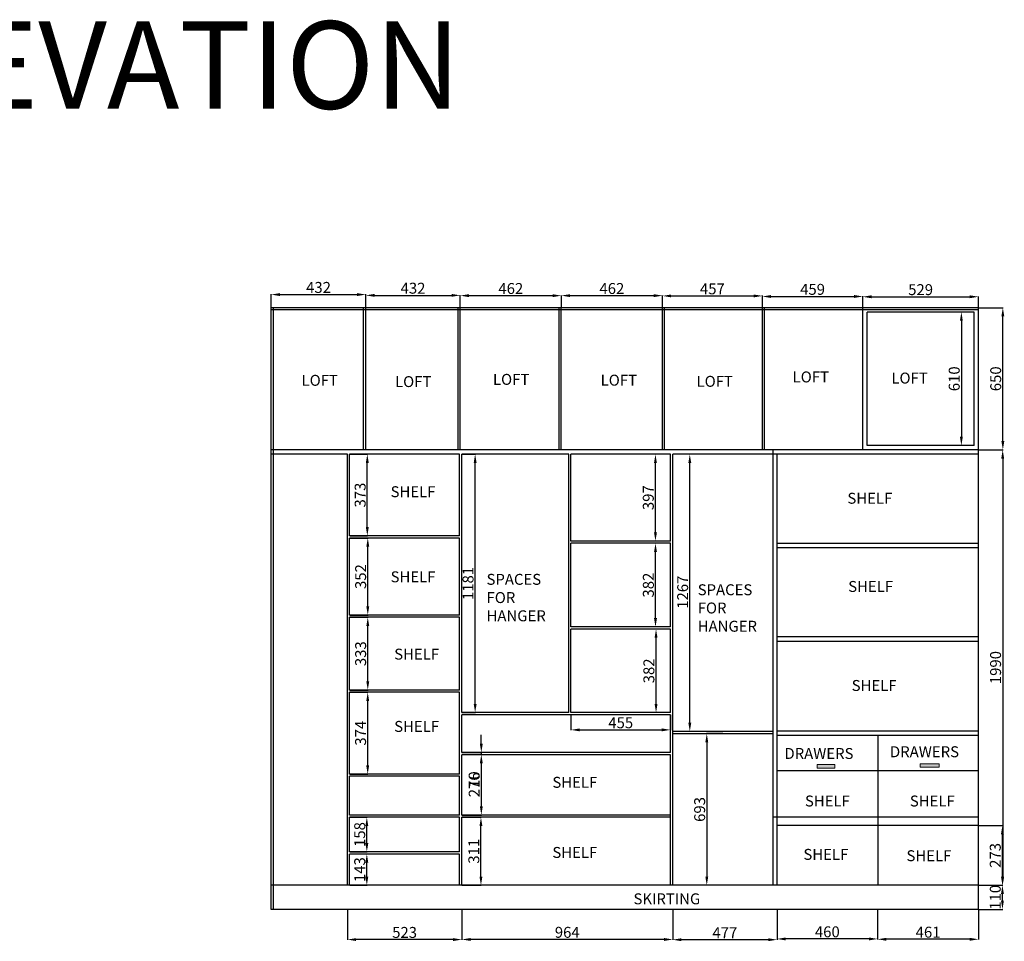
# Model space of a CAD drawing. Units: millimetres. Extents: x 46070 to 59439, y 6883 to 14761.
# Tile 5 of 5: x 54938 to 59439, y 10549 to 14761. Entities that reach past the tile are written whole.
import ezdxf

# ---------------------------------------------------------------- set-up
doc = ezdxf.new("R2010")
doc.units = ezdxf.units.MM
for name, color, linetype, lineweight in [('A-ANNO-DIMS', 2, 'Continuous', 18), ('A-ANNO-TEXT', 7, 'Continuous', 18), ('A-ELEV', 7, 'Continuous', 25), ('A-ELEV-PATT', 8, 'Continuous', 13), ('A-FURN-HDWR', 4, 'Continuous', 18)]:
    doc.layers.add(name, color=color, linetype=linetype, lineweight=lineweight)
doc.styles.get("Standard").update_dxf_attribs({"font": 'arial.ttf'})
doc.dimstyles.new('ISO-25', dxfattribs={"dimtxt": 50, "dimasz": 40, "dimexe": 1.25, "dimexo": 0.625, "dimtad": 1, "dimtxsty": 'Standard', "dimcen": 2.5, "dimadec": 0, "dimazin": 0, "dimtfac": 1, "dimtmove": 0, "dimatfit": 3, "dimfxl": 1, "dimarcsym": 0})

# ---------------------------------------------------------------- blocks, each defined once
blk = doc.blocks.new('*D34')
at = {"layer": 'A-ANNO-DIMS', "color": 0, "lineweight": -2, "transparency": 16777216}
for p, q in [((59321.5, 10805), (59431.6, 10805)), ((59430.3, 10735), (59430.3, 10765)), ((59321.5, 10695), (59431.6, 10695))]:
    blk.add_line(p, q, dxfattribs=at)
at = {"layer": 'A-ANNO-DIMS', "color": 0, "transparency": 16777216}
for points in [[(59423.7, 10765), (59437, 10765), (59430.3, 10805)], [(59423.7, 10735), (59437, 10735), (59430.3, 10695)]]:
    blk.add_solid(points, dxfattribs=at)
at = {"layer": 'Defpoints', "color": 0, "transparency": 16777216}
for p in [(59320.9, 10805), (59430.3, 10805), (59320.9, 10695)]:
    blk.add_point(p, dxfattribs=at)
at = {"layer": 'A-ANNO-DIMS', "color": 0, "transparency": 16777216, "insert": (59404.2, 10750), "char_height": 50, "attachment_point": 5, "rotation": 90}
blk.add_mtext('110', dxfattribs=at)
blk = doc.blocks.new('*D35')
at = {"layer": 'A-ANNO-DIMS', "color": 0, "lineweight": -2, "transparency": 16777216}
for p, q in [((59321.5, 11078), (59431.6, 11078)), ((59430.4, 10845), (59430.4, 11038)), ((59321.5, 10805), (59431.6, 10805))]:
    blk.add_line(p, q, dxfattribs=at)
at = {"layer": 'A-ANNO-DIMS', "color": 0, "transparency": 16777216}
for points in [[(59423.7, 11038), (59437, 11038), (59430.4, 11078)], [(59423.7, 10845), (59437, 10845), (59430.4, 10805)]]:
    blk.add_solid(points, dxfattribs=at)
at = {"layer": 'Defpoints', "color": 0, "transparency": 16777216}
for p in [(59320.9, 11078), (59430.4, 11078), (59320.9, 10805)]:
    blk.add_point(p, dxfattribs=at)
at = {"layer": 'A-ANNO-DIMS', "color": 0, "transparency": 16777216, "insert": (59404.2, 10941.5), "char_height": 50, "attachment_point": 5, "rotation": 90}
blk.add_mtext('273', dxfattribs=at)
blk = doc.blocks.new('*D36')
at = {"layer": 'A-ANNO-DIMS', "color": 0, "lineweight": -2, "transparency": 16777216}
for p, q in [((59321.5, 12795), (59432.9, 12795)), ((59431.6, 12755), (59431.6, 10845)), ((59321.5, 10805), (59432.9, 10805))]:
    blk.add_line(p, q, dxfattribs=at)
at = {"layer": 'A-ANNO-DIMS', "color": 0, "transparency": 16777216}
for points in [[(59424.9, 12755), (59438.3, 12755), (59431.6, 12795)], [(59424.9, 10845), (59438.3, 10845), (59431.6, 10805)]]:
    blk.add_solid(points, dxfattribs=at)
at = {"layer": 'Defpoints', "color": 0, "transparency": 16777216}
for p in [(59320.9, 12795), (59320.9, 10805), (59431.6, 10805)]:
    blk.add_point(p, dxfattribs=at)
at = {"layer": 'A-ANNO-DIMS', "color": 0, "transparency": 16777216, "insert": (59405.5, 11800), "char_height": 50, "attachment_point": 5, "rotation": 90}
blk.add_mtext('1990', dxfattribs=at)
blk = doc.blocks.new('*D37')
at = {"layer": 'A-ANNO-DIMS', "color": 0, "lineweight": -2, "transparency": 16777216}
for p, q in [((58859.9, 10694.3), (58859.9, 10556.8)), ((59320.9, 10694.3), (59320.9, 10556.8)), ((59280.9, 10558.1), (58899.9, 10558.1))]:
    blk.add_line(p, q, dxfattribs=at)
at = {"layer": 'A-ANNO-DIMS', "color": 0, "transparency": 16777216}
for points in [[(58899.9, 10564.8), (58899.9, 10551.4), (58859.9, 10558.1)], [(59280.9, 10564.8), (59280.9, 10551.4), (59320.9, 10558.1)]]:
    blk.add_solid(points, dxfattribs=at)
at = {"layer": 'Defpoints', "color": 0, "transparency": 16777216}
for p in [(58859.9, 10695), (59320.9, 10695), (58859.9, 10558.1)]:
    blk.add_point(p, dxfattribs=at)
at = {"layer": 'A-ANNO-DIMS', "color": 0, "transparency": 16777216, "insert": (59090.4, 10584.2), "char_height": 50, "attachment_point": 5}
blk.add_mtext('461', dxfattribs=at)
blk = doc.blocks.new('*D38')
at = {"layer": 'A-ANNO-DIMS', "color": 0, "lineweight": -2, "transparency": 16777216}
for p, q in [((58399.9, 10694.3), (58399.9, 10558.4)), ((58859.9, 10694.3), (58859.9, 10558.4)), ((58819.9, 10559.6), (58439.9, 10559.6))]:
    blk.add_line(p, q, dxfattribs=at)
at = {"layer": 'A-ANNO-DIMS', "color": 0, "transparency": 16777216}
for points in [[(58439.9, 10566.3), (58439.9, 10553), (58399.9, 10559.6)], [(58819.9, 10566.3), (58819.9, 10553), (58859.9, 10559.6)]]:
    blk.add_solid(points, dxfattribs=at)
at = {"layer": 'Defpoints', "color": 0, "transparency": 16777216}
for p in [(58399.9, 10695), (58859.9, 10695), (58399.9, 10559.6)]:
    blk.add_point(p, dxfattribs=at)
at = {"layer": 'A-ANNO-DIMS', "color": 0, "transparency": 16777216, "insert": (58629.9, 10585.8), "char_height": 50, "attachment_point": 5}
blk.add_mtext('460', dxfattribs=at)
blk = doc.blocks.new('*D39')
at = {"layer": 'A-ANNO-DIMS', "color": 0, "lineweight": -2, "transparency": 16777216}
for p, q in [((57922.9, 10694.3), (57922.9, 10554.9)), ((58399.9, 10694.3), (58399.9, 10554.9)), ((58359.9, 10556.1), (57962.9, 10556.1))]:
    blk.add_line(p, q, dxfattribs=at)
at = {"layer": 'A-ANNO-DIMS', "color": 0, "transparency": 16777216}
for points in [[(57962.9, 10562.8), (57962.9, 10549.4), (57922.9, 10556.1)], [(58359.9, 10562.8), (58359.9, 10549.4), (58399.9, 10556.1)]]:
    blk.add_solid(points, dxfattribs=at)
at = {"layer": 'Defpoints', "color": 0, "transparency": 16777216}
for p in [(57922.9, 10695), (58399.9, 10695), (57922.9, 10556.1)]:
    blk.add_point(p, dxfattribs=at)
at = {"layer": 'A-ANNO-DIMS', "color": 0, "transparency": 16777216, "insert": (58161.4, 10581.7), "char_height": 50, "attachment_point": 5}
blk.add_mtext('477', dxfattribs=at)
blk = doc.blocks.new('*D40')
at = {"layer": 'A-ANNO-DIMS', "color": 0, "lineweight": -2, "transparency": 16777216}
for p, q in [((56958.9, 10694.3), (56958.9, 10556.1)), ((57922.9, 10694.3), (57922.9, 10556.1)), ((57882.9, 10557.3), (56998.9, 10557.3))]:
    blk.add_line(p, q, dxfattribs=at)
at = {"layer": 'A-ANNO-DIMS', "color": 0, "transparency": 16777216}
for points in [[(56998.9, 10564), (56998.9, 10550.6), (56958.9, 10557.3)], [(57882.9, 10564), (57882.9, 10550.6), (57922.9, 10557.3)]]:
    blk.add_solid(points, dxfattribs=at)
at = {"layer": 'Defpoints', "color": 0, "transparency": 16777216}
for p in [(56958.9, 10695), (57922.9, 10695), (56958.9, 10557.3)]:
    blk.add_point(p, dxfattribs=at)
at = {"layer": 'A-ANNO-DIMS', "color": 0, "transparency": 16777216, "insert": (57440.9, 10583.5), "char_height": 50, "attachment_point": 5}
blk.add_mtext('964', dxfattribs=at)
blk = doc.blocks.new('*D41')
at = {"layer": 'A-ANNO-DIMS', "color": 0, "lineweight": -2, "transparency": 16777216}
for p, q in [((56435.9, 10694.3), (56435.9, 10555.5)), ((56958.9, 10694.3), (56958.9, 10555.5)), ((56918.9, 10556.8), (56475.9, 10556.8))]:
    blk.add_line(p, q, dxfattribs=at)
at = {"layer": 'A-ANNO-DIMS', "color": 0, "transparency": 16777216}
for points in [[(56475.9, 10563.4), (56475.9, 10550.1), (56435.9, 10556.8)], [(56918.9, 10563.4), (56918.9, 10550.1), (56958.9, 10556.8)]]:
    blk.add_solid(points, dxfattribs=at)
at = {"layer": 'Defpoints', "color": 0, "transparency": 16777216}
for p in [(56435.9, 10695), (56958.9, 10695), (56435.9, 10556.8)]:
    blk.add_point(p, dxfattribs=at)
at = {"layer": 'A-ANNO-DIMS', "color": 0, "transparency": 16777216, "insert": (56697.4, 10583), "char_height": 50, "attachment_point": 5}
blk.add_mtext('523', dxfattribs=at)
blk = doc.blocks.new('*D43')
at = {"layer": 'A-ANNO-DIMS', "color": 0, "lineweight": -2, "transparency": 16777216}
for p, q in [((59321.5, 13445), (59433.5, 13445)), ((59432.3, 12835), (59432.3, 13405)), ((59321.5, 12795), (59433.5, 12795))]:
    blk.add_line(p, q, dxfattribs=at)
at = {"layer": 'A-ANNO-DIMS', "color": 0, "transparency": 16777216}
for points in [[(59425.6, 13405), (59438.9, 13405), (59432.3, 13445)], [(59425.6, 12835), (59438.9, 12835), (59432.3, 12795)]]:
    blk.add_solid(points, dxfattribs=at)
at = {"layer": 'Defpoints', "color": 0, "transparency": 16777216}
for p in [(59320.9, 13445), (59432.3, 13445), (59320.9, 12795)]:
    blk.add_point(p, dxfattribs=at)
at = {"layer": 'A-ANNO-DIMS', "color": 0, "transparency": 16777216, "insert": (59406.1, 13120), "char_height": 50, "attachment_point": 5, "rotation": 90}
blk.add_mtext('650', dxfattribs=at)
blk = doc.blocks.new('*D44')
at = {"layer": 'A-ANNO-DIMS', "color": 0, "lineweight": -2, "transparency": 16777216}
for p, q in [((59257.7, 13425), (59241.4, 13425)), ((59242.7, 13385), (59242.7, 12855)), ((59257.7, 12815), (59241.4, 12815))]:
    blk.add_line(p, q, dxfattribs=at)
at = {"layer": 'A-ANNO-DIMS', "color": 0, "transparency": 16777216}
for points in [[(59236, 13385), (59249.3, 13385), (59242.7, 13425)], [(59236, 12855), (59249.3, 12855), (59242.7, 12815)]]:
    blk.add_solid(points, dxfattribs=at)
at = {"layer": 'Defpoints', "color": 0, "transparency": 16777216}
for p in [(59258.4, 13425), (59242.7, 12815), (59258.4, 12815)]:
    blk.add_point(p, dxfattribs=at)
at = {"layer": 'A-ANNO-DIMS', "color": 0, "transparency": 16777216, "insert": (59216.5, 13120), "char_height": 50, "attachment_point": 5, "rotation": 90}
blk.add_mtext('610', dxfattribs=at)
blk = doc.blocks.new('*D45')
at = {"layer": 'A-ANNO-DIMS', "color": 0, "lineweight": -2, "transparency": 16777216}
for p, q in [((56087.9, 13445.6), (56087.9, 13506.1)), ((56127.9, 13504.9), (56479.9, 13504.9)), ((56519.9, 13445.6), (56519.9, 13506.1))]:
    blk.add_line(p, q, dxfattribs=at)
at = {"layer": 'A-ANNO-DIMS', "color": 0, "transparency": 16777216}
for points in [[(56127.9, 13511.6), (56127.9, 13498.2), (56087.9, 13504.9)], [(56479.9, 13511.6), (56479.9, 13498.2), (56519.9, 13504.9)]]:
    blk.add_solid(points, dxfattribs=at)
at = {"layer": 'Defpoints', "color": 0, "transparency": 16777216}
for p in [(56519.9, 13504.9), (56087.9, 13445), (56519.9, 13445)]:
    blk.add_point(p, dxfattribs=at)
at = {"layer": 'A-ANNO-DIMS', "color": 0, "transparency": 16777216, "insert": (56303.9, 13531.1), "char_height": 50, "attachment_point": 5}
blk.add_mtext('432', dxfattribs=at)
blk = doc.blocks.new('*D46')
at = {"layer": 'A-ANNO-DIMS', "color": 0, "lineweight": -2, "transparency": 16777216}
for p, q in [((56519.9, 13445.6), (56519.9, 13502.6)), ((56559.9, 13501.3), (56911.9, 13501.3)), ((56951.9, 13445.6), (56951.9, 13502.6))]:
    blk.add_line(p, q, dxfattribs=at)
at = {"layer": 'A-ANNO-DIMS', "color": 0, "transparency": 16777216}
for points in [[(56559.9, 13508), (56559.9, 13494.7), (56519.9, 13501.3)], [(56911.9, 13508), (56911.9, 13494.7), (56951.9, 13501.3)]]:
    blk.add_solid(points, dxfattribs=at)
at = {"layer": 'Defpoints', "color": 0, "transparency": 16777216}
for p in [(56951.9, 13501.3), (56519.9, 13445), (56951.9, 13445)]:
    blk.add_point(p, dxfattribs=at)
at = {"layer": 'A-ANNO-DIMS', "color": 0, "transparency": 16777216, "insert": (56735.9, 13527.5), "char_height": 50, "attachment_point": 5}
blk.add_mtext('432', dxfattribs=at)
blk = doc.blocks.new('*D47')
at = {"layer": 'A-ANNO-DIMS', "color": 0, "lineweight": -2, "transparency": 16777216}
for p, q in [((56951.9, 13445.6), (56951.9, 13501.3)), ((56991.9, 13500), (57373.9, 13500)), ((57413.9, 13445.6), (57413.9, 13501.3))]:
    blk.add_line(p, q, dxfattribs=at)
at = {"layer": 'A-ANNO-DIMS', "color": 0, "transparency": 16777216}
for points in [[(56991.9, 13506.7), (56991.9, 13493.4), (56951.9, 13500)], [(57373.9, 13506.7), (57373.9, 13493.4), (57413.9, 13500)]]:
    blk.add_solid(points, dxfattribs=at)
at = {"layer": 'Defpoints', "color": 0, "transparency": 16777216}
for p in [(57413.9, 13500), (56951.9, 13445), (57413.9, 13445)]:
    blk.add_point(p, dxfattribs=at)
at = {"layer": 'A-ANNO-DIMS', "color": 0, "transparency": 16777216, "insert": (57182.9, 13526.2), "char_height": 50, "attachment_point": 5}
blk.add_mtext('462', dxfattribs=at)
blk = doc.blocks.new('*D48')
at = {"layer": 'A-ANNO-DIMS', "color": 0, "lineweight": -2, "transparency": 16777216}
for p, q in [((57413.9, 13445.6), (57413.9, 13501.3)), ((57453.9, 13500.1), (57835.9, 13500.1)), ((57875.9, 13445.6), (57875.9, 13501.3))]:
    blk.add_line(p, q, dxfattribs=at)
at = {"layer": 'A-ANNO-DIMS', "color": 0, "transparency": 16777216}
for points in [[(57453.9, 13506.7), (57453.9, 13493.4), (57413.9, 13500.1)], [(57835.9, 13506.7), (57835.9, 13493.4), (57875.9, 13500.1)]]:
    blk.add_solid(points, dxfattribs=at)
at = {"layer": 'Defpoints', "color": 0, "transparency": 16777216}
for p in [(57875.9, 13500.1), (57413.9, 13445), (57875.9, 13445)]:
    blk.add_point(p, dxfattribs=at)
at = {"layer": 'A-ANNO-DIMS', "color": 0, "transparency": 16777216, "insert": (57644.9, 13526.2), "char_height": 50, "attachment_point": 5}
blk.add_mtext('462', dxfattribs=at)
blk = doc.blocks.new('*D49')
at = {"layer": 'A-ANNO-DIMS', "color": 0, "lineweight": -2, "transparency": 16777216}
for p, q in [((57875.9, 13445.6), (57875.9, 13500)), ((57915.9, 13498.8), (58292.9, 13498.8)), ((58332.9, 13445.6), (58332.9, 13500))]:
    blk.add_line(p, q, dxfattribs=at)
at = {"layer": 'A-ANNO-DIMS', "color": 0, "transparency": 16777216}
for points in [[(57915.9, 13505.4), (57915.9, 13492.1), (57875.9, 13498.8)], [(58292.9, 13505.4), (58292.9, 13492.1), (58332.9, 13498.8)]]:
    blk.add_solid(points, dxfattribs=at)
at = {"layer": 'Defpoints', "color": 0, "transparency": 16777216}
for p in [(58332.9, 13498.8), (57875.9, 13445), (58332.9, 13445)]:
    blk.add_point(p, dxfattribs=at)
at = {"layer": 'A-ANNO-DIMS', "color": 0, "transparency": 16777216, "insert": (58104.4, 13524.8), "char_height": 50, "attachment_point": 5}
blk.add_mtext('457', dxfattribs=at)
blk = doc.blocks.new('*D50')
at = {"layer": 'A-ANNO-DIMS', "color": 0, "lineweight": -2, "transparency": 16777216}
for p, q in [((58332.9, 13445.6), (58332.9, 13497.4)), ((58372.9, 13496.2), (58751.9, 13496.2)), ((58791.9, 13445.6), (58791.9, 13497.4))]:
    blk.add_line(p, q, dxfattribs=at)
at = {"layer": 'A-ANNO-DIMS', "color": 0, "transparency": 16777216}
for points in [[(58372.9, 13502.9), (58372.9, 13489.5), (58332.9, 13496.2)], [(58751.9, 13502.9), (58751.9, 13489.5), (58791.9, 13496.2)]]:
    blk.add_solid(points, dxfattribs=at)
at = {"layer": 'Defpoints', "color": 0, "transparency": 16777216}
for p in [(58791.9, 13496.2), (58332.9, 13445), (58791.9, 13445)]:
    blk.add_point(p, dxfattribs=at)
at = {"layer": 'A-ANNO-DIMS', "color": 0, "transparency": 16777216, "insert": (58562.4, 13522.3), "char_height": 50, "attachment_point": 5}
blk.add_mtext('459', dxfattribs=at)
blk = doc.blocks.new('*D51')
at = {"layer": 'A-ANNO-DIMS', "color": 0, "lineweight": -2, "transparency": 16777216}
for p, q in [((58791.9, 13445.6), (58791.9, 13496.1)), ((58831.9, 13494.9), (59280.9, 13494.9)), ((59320.9, 13445.6), (59320.9, 13496.1))]:
    blk.add_line(p, q, dxfattribs=at)
at = {"layer": 'A-ANNO-DIMS', "color": 0, "transparency": 16777216}
for points in [[(58831.9, 13501.5), (58831.9, 13488.2), (58791.9, 13494.9)], [(59280.9, 13501.5), (59280.9, 13488.2), (59320.9, 13494.9)]]:
    blk.add_solid(points, dxfattribs=at)
at = {"layer": 'Defpoints', "color": 0, "transparency": 16777216}
for p in [(59320.9, 13494.9), (58791.9, 13445), (59320.9, 13445)]:
    blk.add_point(p, dxfattribs=at)
at = {"layer": 'A-ANNO-DIMS', "color": 0, "transparency": 16777216, "insert": (59056.4, 13521), "char_height": 50, "attachment_point": 5}
blk.add_mtext('529', dxfattribs=at)
blk = doc.blocks.new('*D52')
at = {"layer": 'A-ANNO-DIMS', "color": 0, "lineweight": -2, "transparency": 16777216}
for p, q in [((58151.7, 12775), (57999.9, 12775)), ((58001.1, 11548), (58001.1, 12735)), ((58151.7, 11508), (57999.9, 11508))]:
    blk.add_line(p, q, dxfattribs=at)
at = {"layer": 'A-ANNO-DIMS', "color": 0, "transparency": 16777216}
for points in [[(57994.5, 12735), (58007.8, 12735), (58001.1, 12775)], [(57994.5, 11548), (58007.8, 11548), (58001.1, 11508)]]:
    blk.add_solid(points, dxfattribs=at)
at = {"layer": 'Defpoints', "color": 0, "transparency": 16777216}
for p in [(58001.1, 12775), (58152.4, 12775), (58152.4, 11508)]:
    blk.add_point(p, dxfattribs=at)
at = {"layer": 'A-ANNO-DIMS', "color": 0, "transparency": 16777216, "insert": (57975, 12144.6), "char_height": 50, "attachment_point": 5, "rotation": 90}
blk.add_mtext('1267', dxfattribs=at)
blk = doc.blocks.new('*D53')
at = {"layer": 'A-ANNO-DIMS', "color": 0, "lineweight": -2, "transparency": 16777216}
for p, q in [((58151.7, 11498), (58077.6, 11498)), ((58078.8, 11458), (58078.8, 10845)), ((58151.7, 10805), (58077.6, 10805))]:
    blk.add_line(p, q, dxfattribs=at)
at = {"layer": 'A-ANNO-DIMS', "color": 0, "transparency": 16777216}
for points in [[(58072.2, 11458), (58085.5, 11458), (58078.8, 11498)], [(58072.2, 10845), (58085.5, 10845), (58078.8, 10805)]]:
    blk.add_solid(points, dxfattribs=at)
at = {"layer": 'Defpoints', "color": 0, "transparency": 16777216}
for p in [(58152.4, 11498), (58078.8, 10805), (58152.4, 10805)]:
    blk.add_point(p, dxfattribs=at)
at = {"layer": 'A-ANNO-DIMS', "color": 0, "transparency": 16777216, "insert": (58052.7, 11151.5), "char_height": 50, "attachment_point": 5, "rotation": 90}
blk.add_mtext('693', dxfattribs=at)
blk = doc.blocks.new('*D54')
at = {"layer": 'A-ANNO-DIMS', "color": 0, "lineweight": -2, "transparency": 16777216}
for p, q in [((56959.5, 11402), (57049.4, 11402)), ((57048.2, 11166), (57048.2, 11362)), ((56959.5, 11126), (57049.4, 11126))]:
    blk.add_line(p, q, dxfattribs=at)
at = {"layer": 'A-ANNO-DIMS', "color": 0, "transparency": 16777216}
for points in [[(57041.5, 11362), (57054.8, 11362), (57048.2, 11402)], [(57041.5, 11166), (57054.8, 11166), (57048.2, 11126)]]:
    blk.add_solid(points, dxfattribs=at)
at = {"layer": 'Defpoints', "color": 0, "transparency": 16777216}
for p in [(56958.9, 11402), (57048.2, 11402), (56958.9, 11126)]:
    blk.add_point(p, dxfattribs=at)
at = {"layer": 'A-ANNO-DIMS', "color": 0, "transparency": 16777216, "insert": (57022, 11264), "char_height": 50, "attachment_point": 5, "rotation": 90}
blk.add_mtext('276', dxfattribs=at)
blk = doc.blocks.new('*D55')
at = {"layer": 'A-ANNO-DIMS', "color": 0, "lineweight": -2, "transparency": 16777216}
for p, q in [((56959.5, 12775), (57021.1, 12775)), ((57019.8, 11634), (57019.8, 12735)), ((56959.5, 11594), (57021.1, 11594))]:
    blk.add_line(p, q, dxfattribs=at)
at = {"layer": 'A-ANNO-DIMS', "color": 0, "transparency": 16777216}
for points in [[(57013.2, 12735), (57026.5, 12735), (57019.8, 12775)], [(57013.2, 11634), (57026.5, 11634), (57019.8, 11594)]]:
    blk.add_solid(points, dxfattribs=at)
at = {"layer": 'Defpoints', "color": 0, "transparency": 16777216}
for p in [(56958.9, 12775), (57019.8, 12775), (56958.9, 11594)]:
    blk.add_point(p, dxfattribs=at)
at = {"layer": 'A-ANNO-DIMS', "color": 0, "transparency": 16777216, "insert": (56993.7, 12184.5), "char_height": 50, "attachment_point": 5, "rotation": 90}
blk.add_mtext('1181', dxfattribs=at)
blk = doc.blocks.new('*D56')
at = {"layer": 'A-ANNO-DIMS', "color": 0, "lineweight": -2, "transparency": 16777216}
for p, q in [((57457.9, 11583.3), (57457.9, 11514)), ((57912.9, 11583.3), (57912.9, 11514)), ((57497.9, 11515.3), (57872.9, 11515.3))]:
    blk.add_line(p, q, dxfattribs=at)
at = {"layer": 'A-ANNO-DIMS', "color": 0, "transparency": 16777216}
for points in [[(57497.9, 11522), (57497.9, 11508.6), (57457.9, 11515.3)], [(57872.9, 11522), (57872.9, 11508.6), (57912.9, 11515.3)]]:
    blk.add_solid(points, dxfattribs=at)
at = {"layer": 'Defpoints', "color": 0, "transparency": 16777216}
for p in [(57457.9, 11584), (57912.9, 11584), (57912.9, 11515.3)]:
    blk.add_point(p, dxfattribs=at)
at = {"layer": 'A-ANNO-DIMS', "color": 0, "transparency": 16777216, "insert": (57685.4, 11541.3), "char_height": 50, "attachment_point": 5}
blk.add_mtext('455', dxfattribs=at)
blk = doc.blocks.new('*D57')
at = {"layer": 'A-ANNO-DIMS', "color": 0, "lineweight": -2, "transparency": 16777216}
for p, q in [((57047.9, 11452), (57047.9, 11492)), ((56959.5, 11412), (57049.2, 11412)), ((56959.5, 11402), (57049.2, 11402)), ((57047.9, 11412), (57047.9, 11402)), ((57047.9, 11362), (57047.9, 11254))]:
    blk.add_line(p, q, dxfattribs=at)
at = {"layer": 'A-ANNO-DIMS', "color": 0, "transparency": 16777216}
for points in [[(57041.2, 11452), (57054.6, 11452), (57047.9, 11412)], [(57041.2, 11362), (57054.6, 11362), (57047.9, 11402)]]:
    blk.add_solid(points, dxfattribs=at)
at = {"layer": 'Defpoints', "color": 0, "transparency": 16777216}
for p in [(56958.9, 11412), (56958.9, 11402), (57047.9, 11402)]:
    blk.add_point(p, dxfattribs=at)
at = {"layer": 'A-ANNO-DIMS', "color": 0, "transparency": 16777216, "insert": (57021.8, 11288), "char_height": 50, "attachment_point": 5, "rotation": 90}
blk.add_mtext('10', dxfattribs=at)
blk = doc.blocks.new('*D58')
at = {"layer": 'A-ANNO-DIMS', "color": 0, "lineweight": -2, "transparency": 16777216}
for p, q in [((57912.2, 11976), (57845.6, 11976)), ((57846.8, 11634), (57846.8, 11936)), ((57912.2, 11594), (57845.6, 11594))]:
    blk.add_line(p, q, dxfattribs=at)
at = {"layer": 'A-ANNO-DIMS', "color": 0, "transparency": 16777216}
for points in [[(57840.1, 11936), (57853.5, 11936), (57846.8, 11976)], [(57840.1, 11634), (57853.5, 11634), (57846.8, 11594)]]:
    blk.add_solid(points, dxfattribs=at)
at = {"layer": 'Defpoints', "color": 0, "transparency": 16777216}
for p in [(57846.8, 11976), (57912.9, 11976), (57912.9, 11594)]:
    blk.add_point(p, dxfattribs=at)
at = {"layer": 'A-ANNO-DIMS', "color": 0, "transparency": 16777216, "insert": (57820.6, 11785), "char_height": 50, "attachment_point": 5, "rotation": 90}
blk.add_mtext('382', dxfattribs=at)
blk = doc.blocks.new('*D59')
at = {"layer": 'A-ANNO-DIMS', "color": 0, "lineweight": -2, "transparency": 16777216}
for p, q in [((57912.2, 12368), (57843.1, 12368)), ((57844.3, 12026), (57844.3, 12328)), ((57912.2, 11986), (57843.1, 11986))]:
    blk.add_line(p, q, dxfattribs=at)
at = {"layer": 'A-ANNO-DIMS', "color": 0, "transparency": 16777216}
for points in [[(57837.6, 12328), (57851, 12328), (57844.3, 12368)], [(57837.6, 12026), (57851, 12026), (57844.3, 11986)]]:
    blk.add_solid(points, dxfattribs=at)
at = {"layer": 'Defpoints', "color": 0, "transparency": 16777216}
for p in [(57844.3, 12368), (57912.9, 12368), (57912.9, 11986)]:
    blk.add_point(p, dxfattribs=at)
at = {"layer": 'A-ANNO-DIMS', "color": 0, "transparency": 16777216, "insert": (57818.1, 12177), "char_height": 50, "attachment_point": 5, "rotation": 90}
blk.add_mtext('382', dxfattribs=at)
blk = doc.blocks.new('*D60')
at = {"layer": 'A-ANNO-DIMS', "color": 0, "lineweight": -2, "transparency": 16777216}
for p, q in [((57912.2, 12775), (57842.9, 12775)), ((57844.1, 12418), (57844.1, 12735)), ((57912.2, 12378), (57842.9, 12378))]:
    blk.add_line(p, q, dxfattribs=at)
at = {"layer": 'A-ANNO-DIMS', "color": 0, "transparency": 16777216}
for points in [[(57837.4, 12735), (57850.8, 12735), (57844.1, 12775)], [(57837.4, 12418), (57850.8, 12418), (57844.1, 12378)]]:
    blk.add_solid(points, dxfattribs=at)
at = {"layer": 'Defpoints', "color": 0, "transparency": 16777216}
for p in [(57844.1, 12775), (57912.9, 12775), (57912.9, 12378)]:
    blk.add_point(p, dxfattribs=at)
at = {"layer": 'A-ANNO-DIMS', "color": 0, "transparency": 16777216, "insert": (57817.9, 12576.5), "char_height": 50, "attachment_point": 5, "rotation": 90}
blk.add_mtext('397', dxfattribs=at)
blk = doc.blocks.new('*D61')
at = {"layer": 'A-ANNO-DIMS', "color": 0, "lineweight": -2, "transparency": 16777216}
for p, q in [((56446.5, 10948), (56526, 10948)), ((56524.7, 10845), (56524.7, 10908)), ((56446.5, 10805), (56526, 10805))]:
    blk.add_line(p, q, dxfattribs=at)
at = {"layer": 'A-ANNO-DIMS', "color": 0, "transparency": 16777216}
for points in [[(56518.1, 10908), (56531.4, 10908), (56524.7, 10948)], [(56518.1, 10845), (56531.4, 10845), (56524.7, 10805)]]:
    blk.add_solid(points, dxfattribs=at)
at = {"layer": 'Defpoints', "color": 0, "transparency": 16777216}
for p in [(56445.9, 10948), (56524.7, 10948), (56445.9, 10805)]:
    blk.add_point(p, dxfattribs=at)
at = {"layer": 'A-ANNO-DIMS', "color": 0, "transparency": 16777216, "insert": (56498.6, 10876.5), "char_height": 50, "attachment_point": 5, "rotation": 90}
blk.add_mtext('143', dxfattribs=at)
blk = doc.blocks.new('*D62')
at = {"layer": 'A-ANNO-DIMS', "color": 0, "lineweight": -2, "transparency": 16777216}
for p, q in [((56959.5, 11116), (57047.6, 11116)), ((57046.4, 10845), (57046.4, 11076)), ((56959.5, 10805), (57047.6, 10805))]:
    blk.add_line(p, q, dxfattribs=at)
at = {"layer": 'A-ANNO-DIMS', "color": 0, "transparency": 16777216}
for points in [[(57039.7, 11076), (57053, 11076), (57046.4, 11116)], [(57039.7, 10845), (57053, 10845), (57046.4, 10805)]]:
    blk.add_solid(points, dxfattribs=at)
at = {"layer": 'Defpoints', "color": 0, "transparency": 16777216}
for p in [(56958.9, 11116), (57046.4, 11116), (56958.9, 10805)]:
    blk.add_point(p, dxfattribs=at)
at = {"layer": 'A-ANNO-DIMS', "color": 0, "transparency": 16777216, "insert": (57020.2, 10960.5), "char_height": 50, "attachment_point": 5, "rotation": 90}
blk.add_mtext('311', dxfattribs=at)
blk = doc.blocks.new('*D63')
at = {"layer": 'A-ANNO-DIMS', "color": 0, "lineweight": -2, "transparency": 16777216}
for p, q in [((56446.5, 11116), (56526, 11116)), ((56524.7, 10998), (56524.7, 11076)), ((56446.5, 10958), (56526, 10958))]:
    blk.add_line(p, q, dxfattribs=at)
at = {"layer": 'A-ANNO-DIMS', "color": 0, "transparency": 16777216}
for points in [[(56518.1, 11076), (56531.4, 11076), (56524.7, 11116)], [(56518.1, 10998), (56531.4, 10998), (56524.7, 10958)]]:
    blk.add_solid(points, dxfattribs=at)
at = {"layer": 'Defpoints', "color": 0, "transparency": 16777216}
for p in [(56445.9, 11116), (56524.7, 11116), (56445.9, 10958)]:
    blk.add_point(p, dxfattribs=at)
at = {"layer": 'A-ANNO-DIMS', "color": 0, "transparency": 16777216, "insert": (56498.6, 11037), "char_height": 50, "attachment_point": 5, "rotation": 90}
blk.add_mtext('158', dxfattribs=at)
blk = doc.blocks.new('*D64')
at = {"layer": 'A-ANNO-DIMS', "color": 0, "lineweight": -2, "transparency": 16777216}
for p, q in [((56446.5, 12775), (56528.1, 12775)), ((56526.8, 12442), (56526.8, 12735)), ((56446.5, 12402), (56528.1, 12402))]:
    blk.add_line(p, q, dxfattribs=at)
at = {"layer": 'A-ANNO-DIMS', "color": 0, "transparency": 16777216}
for points in [[(56520.2, 12735), (56533.5, 12735), (56526.8, 12775)], [(56520.2, 12442), (56533.5, 12442), (56526.8, 12402)]]:
    blk.add_solid(points, dxfattribs=at)
at = {"layer": 'Defpoints', "color": 0, "transparency": 16777216}
for p in [(56445.9, 12775), (56526.8, 12775), (56445.9, 12402)]:
    blk.add_point(p, dxfattribs=at)
at = {"layer": 'A-ANNO-DIMS', "color": 0, "transparency": 16777216, "insert": (56500.6, 12588.5), "char_height": 50, "attachment_point": 5, "rotation": 90}
blk.add_mtext('373', dxfattribs=at)
blk = doc.blocks.new('*D65')
at = {"layer": 'A-ANNO-DIMS', "color": 0, "lineweight": -2, "transparency": 16777216}
for p, q in [((56446.5, 12392), (56530.3, 12392)), ((56529, 12080), (56529, 12352)), ((56446.5, 12040), (56530.3, 12040))]:
    blk.add_line(p, q, dxfattribs=at)
at = {"layer": 'A-ANNO-DIMS', "color": 0, "transparency": 16777216}
for points in [[(56522.4, 12352), (56535.7, 12352), (56529, 12392)], [(56522.4, 12080), (56535.7, 12080), (56529, 12040)]]:
    blk.add_solid(points, dxfattribs=at)
at = {"layer": 'Defpoints', "color": 0, "transparency": 16777216}
for p in [(56445.9, 12392), (56529, 12392), (56445.9, 12040)]:
    blk.add_point(p, dxfattribs=at)
at = {"layer": 'A-ANNO-DIMS', "color": 0, "transparency": 16777216, "insert": (56502.9, 12216), "char_height": 50, "attachment_point": 5, "rotation": 90}
blk.add_mtext('352', dxfattribs=at)
blk = doc.blocks.new('*D66')
at = {"layer": 'A-ANNO-DIMS', "color": 0, "lineweight": -2, "transparency": 16777216}
for p, q in [((56446.5, 12030), (56530.3, 12030)), ((56529, 11737), (56529, 11990)), ((56446.5, 11697), (56530.3, 11697))]:
    blk.add_line(p, q, dxfattribs=at)
at = {"layer": 'A-ANNO-DIMS', "color": 0, "transparency": 16777216}
for points in [[(56522.4, 11990), (56535.7, 11990), (56529, 12030)], [(56522.4, 11737), (56535.7, 11737), (56529, 11697)]]:
    blk.add_solid(points, dxfattribs=at)
at = {"layer": 'Defpoints', "color": 0, "transparency": 16777216}
for p in [(56445.9, 12030), (56529, 12030), (56445.9, 11697)]:
    blk.add_point(p, dxfattribs=at)
at = {"layer": 'A-ANNO-DIMS', "color": 0, "transparency": 16777216, "insert": (56502.9, 11863.5), "char_height": 50, "attachment_point": 5, "rotation": 90}
blk.add_mtext('333', dxfattribs=at)
blk = doc.blocks.new('*D67')
at = {"layer": 'A-ANNO-DIMS', "color": 0, "lineweight": -2, "transparency": 16777216}
for p, q in [((56446.5, 11687), (56529.9, 11687)), ((56528.7, 11353), (56528.7, 11647)), ((56446.5, 11313), (56529.9, 11313))]:
    blk.add_line(p, q, dxfattribs=at)
at = {"layer": 'A-ANNO-DIMS', "color": 0, "transparency": 16777216}
for points in [[(56522, 11647), (56535.4, 11647), (56528.7, 11687)], [(56522, 11353), (56535.4, 11353), (56528.7, 11313)]]:
    blk.add_solid(points, dxfattribs=at)
at = {"layer": 'Defpoints', "color": 0, "transparency": 16777216}
for p in [(56445.9, 11687), (56528.7, 11687), (56445.9, 11313)]:
    blk.add_point(p, dxfattribs=at)
at = {"layer": 'A-ANNO-DIMS', "color": 0, "transparency": 16777216, "insert": (56502.5, 11500), "char_height": 50, "attachment_point": 5, "rotation": 90}
blk.add_mtext('374', dxfattribs=at)

msp = doc.modelspace()

# ---------------------------------------------------------------- hatches: boundary and pattern name
at = {"layer": 'A-ELEV-PATT'}
h = msp.add_hatch(color=256, dxfattribs=at)
h.dxf.hatch_style = 1
h.paths.add_polyline_path([(59141.9, 11359.789), (59054.18, 11359.789), (59054.18, 11344.587), (59141.9, 11344.587)])
h.paths.add_polyline_path([(58664.208, 11357.753), (58583.077, 11357.753), (58583.077, 11341.031), (58664.208, 11341.031)])

# ---------------------------------------------------------------- linework, layer by layer
at = {"layer": 'A-ELEV'}
for p, q in [((56087.85, 10694.958), (56087.85, 13444.958)), ((59320.85, 13444.958), (56087.85, 13444.958)), ((59320.85, 13434.958), (56087.85, 13434.958)), ((56097.85, 10694.958), (56097.85, 13444.958)), ((56509.85, 12794.958), (56509.85, 13444.958)), ((56519.85, 12794.958), (56519.85, 13444.958)), ((56941.85, 12794.958), (56941.85, 13444.958)), ((56951.85, 12794.958), (56951.85, 13444.958)), ((57403.85, 12794.958), (57403.85, 13444.958)), ((57413.85, 12794.958), (57413.85, 13444.958)), ((57875.85, 12794.958), (57875.85, 13444.958)), ((57885.85, 12794.958), (57885.85, 13444.958)), ((58332.85, 12794.958), (58332.85, 13444.958)), ((58342.85, 12794.958), (58342.85, 13444.958)), ((58791.85, 12794.958), (58791.85, 13444.958)), ((59300.85, 13424.958), (58811.85, 13424.958)), ((58811.85, 12814.958), (58811.85, 13424.958)), ((59300.85, 12814.958), (59300.85, 13424.958)), ((59320.85, 10804.958), (59320.85, 13444.958)), ((59320.85, 12794.958), (56087.85, 12794.958)), ((58381.85, 10804.958), (58381.85, 12794.958)), ((59300.85, 12814.958), (58811.85, 12814.958)), ((56435.85, 12774.958), (56087.85, 12774.958)), ((56435.85, 10804.958), (56435.85, 12774.958)), ((56948.85, 12774.958), (56445.85, 12774.958)), ((56445.85, 12401.958), (56445.85, 12774.958)), ((56948.85, 12401.958), (56948.85, 12774.958)), ((56958.85, 11593.958), (56958.85, 12774.958)), ((57447.85, 12774.958), (56958.85, 12774.958)), ((57447.85, 11593.958), (57447.85, 12774.958)), ((57912.85, 12774.958), (57457.85, 12774.958)), ((57457.85, 12377.958), (57457.85, 12774.958)), ((57912.85, 12377.958), (57912.85, 12774.958)), ((57922.85, 10804.958), (57922.85, 12774.958)), ((59320.85, 12774.958), (57922.85, 12774.958)), ((58399.85, 10804.958), (58399.85, 12774.958)), ((56948.85, 12401.958), (56445.85, 12401.958)), ((56948.85, 12391.958), (56445.85, 12391.958)), ((56445.85, 12039.958), (56445.85, 12391.958)), ((56948.85, 12039.958), (56948.85, 12391.958)), ((57912.85, 12377.958), (57457.85, 12377.958)), ((57912.85, 12367.958), (57457.85, 12367.958)), ((57457.85, 11985.958), (57457.85, 12367.958)), ((57912.85, 11985.958), (57912.85, 12367.958)), ((59320.85, 12366.958), (58399.85, 12366.958)), ((59320.85, 12346.958), (58399.85, 12346.958)), ((56948.85, 12039.958), (56445.85, 12039.958)), ((56948.85, 12029.958), (56445.85, 12029.958)), ((56445.85, 11696.958), (56445.85, 12029.958)), ((56948.85, 11696.958), (56948.85, 12029.958)), ((57912.85, 11985.958), (57457.85, 11985.958)), ((57457.85, 11593.958), (57457.85, 11975.958)), ((57912.85, 11975.958), (57457.85, 11975.958)), ((57912.85, 11593.958), (57912.85, 11975.958)), ((59320.85, 11939.958), (58399.85, 11939.958)), ((59320.85, 11919.958), (58399.85, 11919.958)), ((56948.85, 11696.958), (56445.85, 11696.958)), ((56948.85, 11686.958), (56445.85, 11686.958)), ((56445.85, 11312.958), (56445.85, 11686.958)), ((56948.85, 11312.958), (56948.85, 11686.958)), ((57447.85, 11593.958), (56958.85, 11593.958)), ((57912.85, 11583.958), (56958.85, 11583.958)), ((56958.85, 11411.958), (56958.85, 11583.958)), ((57912.85, 11593.958), (57457.85, 11593.958)), ((57912.85, 11411.958), (57912.85, 11583.958)), ((58381.85, 11507.958), (57922.85, 11507.958)), ((58381.85, 11497.958), (57922.85, 11497.958)), ((59320.85, 11508.958), (58399.85, 11508.958)), ((59320.85, 11488.958), (58399.85, 11488.958)), ((58860.35, 11488.958), (58860.35, 10804.958)), ((57912.85, 11411.958), (56958.85, 11411.958)), ((57912.85, 11401.958), (56958.85, 11401.958)), ((56958.85, 11125.958), (56958.85, 11401.958)), ((57912.85, 10804.958), (57912.85, 11401.958)), ((56948.85, 11312.958), (56445.85, 11312.958)), ((56445.85, 11125.958), (56445.85, 11302.958)), ((56948.85, 11302.958), (56445.85, 11302.958)), ((56948.85, 11125.958), (56948.85, 11302.958)), ((59320.85, 11327.958), (58399.85, 11327.958)), ((56948.85, 11125.958), (56445.85, 11125.958)), ((57912.85, 11125.958), (56958.85, 11125.958)), ((56948.85, 11115.958), (56445.85, 11115.958)), ((56445.85, 10957.958), (56445.85, 11115.958)), ((56948.85, 10957.958), (56948.85, 11115.958)), ((56958.85, 10804.958), (56958.85, 11115.958)), ((57912.85, 11115.958), (56958.85, 11115.958)), ((59320.85, 11115.958), (58381.85, 11115.958)), ((59320.85, 11077.958), (58399.85, 11077.958)), ((56948.85, 10957.958), (56445.85, 10957.958)), ((56948.85, 10947.958), (56445.85, 10947.958)), ((56445.85, 10804.958), (56445.85, 10947.958)), ((56948.85, 10804.958), (56948.85, 10947.958)), ((59320.85, 10804.958), (56087.85, 10804.958)), ((59320.85, 10694.958), (59320.85, 10804.958)), ((57922.85, 10694.958), (56087.85, 10694.958)), ((59320.85, 10694.958), (57922.85, 10694.958))]:
    msp.add_line(p, q, dxfattribs=at)
at = {"layer": 'A-FURN-HDWR'}
for points in [[(58583.077, 11357.753), (58664.208, 11357.753), (58664.208, 11341.031), (58583.077, 11341.031)], [(59054.18, 11359.789), (59141.9, 11359.789), (59141.9, 11344.587), (59054.18, 11344.587)]]:
    msp.add_lwpolyline(points, close=True, dxfattribs=at)

# ---------------------------------------------------------------- texts
at = {"layer": 'A-ANNO-TEXT', "attachment_point": 1}
for s, width, insert, char_height in [('MBR WARDROBE ELEVATION', 11748.56084, (49726.408, 14754.198), 400), ('LOFT', 502.17574, (58471.184, 13153.476), 50), ('LOFT', 502.17574, (58922.714, 13148.189), 50), ('LOFT', 502.17574, (56226.344, 13137.897), 50), ('LOFT', 502.17574, (56653.574, 13132.143), 50), ('LOFT', 502.17574, (57101.339, 13142.346), 50), ('LOFT', 502.17574, (57593.581, 13138.646), 50), ('LOFT', 502.17574, (58032.157, 13133.359), 50), ('SHELF', 502.17574, (56633.294, 12628.86), 50), ('SHELF', 502.17574, (58721.661, 12598.96), 50), ('SHELF', 502.17574, (56633.294, 12239.869), 50), ('SPACES  FOR HANGER ', 303.83076, (57071.897, 12228.339), 50), ('SPACES  FOR HANGER ', 303.83076, (58037.313, 12180.74), 50), ('SHELF', 502.17574, (58725.167, 12195.795), 50), ('SHELF', 502.17574, (56649.665, 11886.442), 50), ('SHELF', 502.17574, (58741.213, 11743.227), 50), ('SHELF', 502.17574, (56649.665, 11556.065), 50), ('DRAWERS', 502.17574, (58433.658, 11432.338), 50), ('DRAWERS', 502.17574, (58916.126, 11440.32), 50), ('SHELF', 502.17574, (57372.896, 11300.606), 50), ('SHELF', 502.17574, (58527.576, 11215.152), 50), ('SHELF', 502.17574, (59007.112, 11215.152), 50), ('SHELF', 502.17574, (57372.896, 10980.052), 50), ('SHELF', 502.17574, (58520.516, 10971.193), 50), ('SHELF', 502.17574, (58991.627, 10965.111), 50), ('SKIRTING ', 502.17574, (57743.661, 10768.085), 50)]:
    msp.add_mtext_dynamic_manual_height_columns(s, width=width, gutter_width=12.5, heights=[0], dxfattribs=dict(at, insert=insert, char_height=char_height))

# ---------------------------------------------------------------- dimensions: what is measured, and where the dimension line sits
at = {"layer": 'A-ANNO-DIMS'}
for base, p1, p2, picture, middle in [((56519.85, 13504.89), (56087.85, 13444.958), (56519.85, 13444.958), '*D45', (56303.85, 13531.06)), ((56951.85, 13501.335), (56519.85, 13444.958), (56951.85, 13444.958), '*D46', (56735.85, 13527.505)), ((57413.85, 13500.03), (56951.85, 13444.958), (57413.85, 13444.958), '*D47', (57182.85, 13526.183)), ((57875.85, 13500.062), (57413.85, 13444.958), (57875.85, 13444.958), '*D48', (57644.85, 13526.216)), ((58332.85, 13498.757), (57875.85, 13444.958), (58332.85, 13444.958), '*D49', (58104.35, 13524.809)), ((58791.85, 13496.186), (58332.85, 13444.958), (58791.85, 13444.958), '*D50', (58562.35, 13522.34)), ((59320.85, 13494.868), (58791.85, 13444.958), (59320.85, 13444.958), '*D51', (59056.35, 13521.021)), ((57912.85, 11515.293), (57457.85, 11583.958), (57912.85, 11583.958), '*D56', (57685.35, 11541.344)), ((56435.85, 10556.78), (56958.85, 10694.958), (56435.85, 10694.958), '*D41', (56697.35, 10582.95)), ((56958.85, 10557.316), (57922.85, 10694.958), (56958.85, 10694.958), '*D40', (57440.85, 10583.47)), ((57922.85, 10556.114), (58399.85, 10694.958), (57922.85, 10694.958), '*D39', (58161.35, 10581.739)), ((58399.85, 10559.646), (58859.85, 10694.958), (58399.85, 10694.958), '*D38', (58629.85, 10585.799)), ((58859.85, 10558.092), (59320.85, 10694.958), (58859.85, 10694.958), '*D37', (59090.35, 10584.246))]:
    dim = msp.add_linear_dim(base=base, p1=p1, p2=p2, dimstyle='ISO-25', override={"dimclrd": 0, "dimclre": 0, "dimclrt": 0}, dxfattribs=at)
    dim.commit()
    dim.dimension.update_dxf_attribs({"geometry": picture, "text_midpoint": middle})
for base, p1, p2, picture, middle in [((59242.659, 12814.958), (59258.353, 13424.958), (59258.353, 12814.958), '*D44', (59242.659, 13119.958)), ((57019.843, 12774.958), (56958.85, 11593.958), (56958.85, 12774.958), '*D55', (57019.843, 12184.458)), ((58001.135, 12774.958), (58152.35, 11507.958), (58152.35, 12774.958), '*D52', (58001.135, 12144.585))]:
    dim = msp.add_linear_dim(base=base, p1=p1, p2=p2, angle=90, dimstyle='ISO-25', override={"dimclrd": 0, "dimclre": 0, "dimclrt": 0}, dxfattribs=at)
    dim.commit()
    dim.dimension.update_dxf_attribs({"geometry": picture, "text_midpoint": middle, "dimtype": 160})
for base, p1, p2, picture, middle in [((59432.279, 13444.958), (59320.85, 12794.958), (59320.85, 13444.958), '*D43', (59406.126, 13119.958)), ((59431.609, 10804.958), (59320.85, 12794.958), (59320.85, 10804.958), '*D36', (59405.455, 11799.958)), ((56526.818, 12774.958), (56445.85, 12401.958), (56445.85, 12774.958), '*D64', (56500.647, 12588.458)), ((57844.102, 12774.958), (57912.85, 12377.958), (57912.85, 12774.958), '*D60', (57817.931, 12576.458)), ((56529.031, 12391.958), (56445.85, 12039.958), (56445.85, 12391.958), '*D65', (56502.86, 12215.958)), ((57844.305, 12367.958), (57912.85, 11985.958), (57912.85, 12367.958), '*D59', (57818.134, 12176.958)), ((57846.813, 11975.958), (57912.85, 11593.958), (57912.85, 11975.958), '*D58', (57820.642, 11784.958)), ((56528.696, 11686.958), (56445.85, 11312.958), (56445.85, 11686.958), '*D67', (56502.526, 11499.958)), ((57047.906, 11401.958), (56958.85, 11411.958), (56958.85, 11401.958), '*D57', (57021.752, 11287.96)), ((58078.849, 10804.958), (58152.35, 11497.958), (58152.35, 10804.958), '*D53', (58052.678, 11151.458)), ((57048.17, 11401.958), (56958.85, 11125.958), (56958.85, 11401.958), '*D54', (57022.016, 11263.958)), ((56524.748, 11115.958), (56445.85, 10957.958), (56445.85, 11115.958), '*D63', (56498.594, 11036.958)), ((57046.376, 11115.958), (56958.85, 10804.958), (56958.85, 11115.958), '*D62', (57020.205, 10960.458)), ((59430.359, 11077.958), (59320.85, 10804.958), (59320.85, 11077.958), '*D35', (59404.188, 10941.458)), ((56524.745, 10947.958), (56445.85, 10804.958), (56445.85, 10947.958), '*D61', (56498.574, 10876.458)), ((59430.317, 10804.958), (59320.85, 10694.958), (59320.85, 10804.958), '*D34', (59404.163, 10749.958))]:
    dim = msp.add_linear_dim(base=base, p1=p1, p2=p2, angle=90, dimstyle='ISO-25', override={"dimclrd": 0, "dimclre": 0, "dimclrt": 0}, dxfattribs=at)
    dim.commit()
    dim.dimension.update_dxf_attribs({"geometry": picture, "text_midpoint": middle})
dim = msp.add_aligned_dim(p1=(56445.85, 11696.958), p2=(56445.85, 12029.958), distance=-83.175, dimstyle='ISO-25', override={"dimclrd": 0, "dimclre": 0, "dimclrt": 0}, dxfattribs=at)
dim.commit()
dim.dimension.update_dxf_attribs({"geometry": '*D66', "text_midpoint": (56502.855, 11863.458)})

doc.saveas('drawing.dxf')
